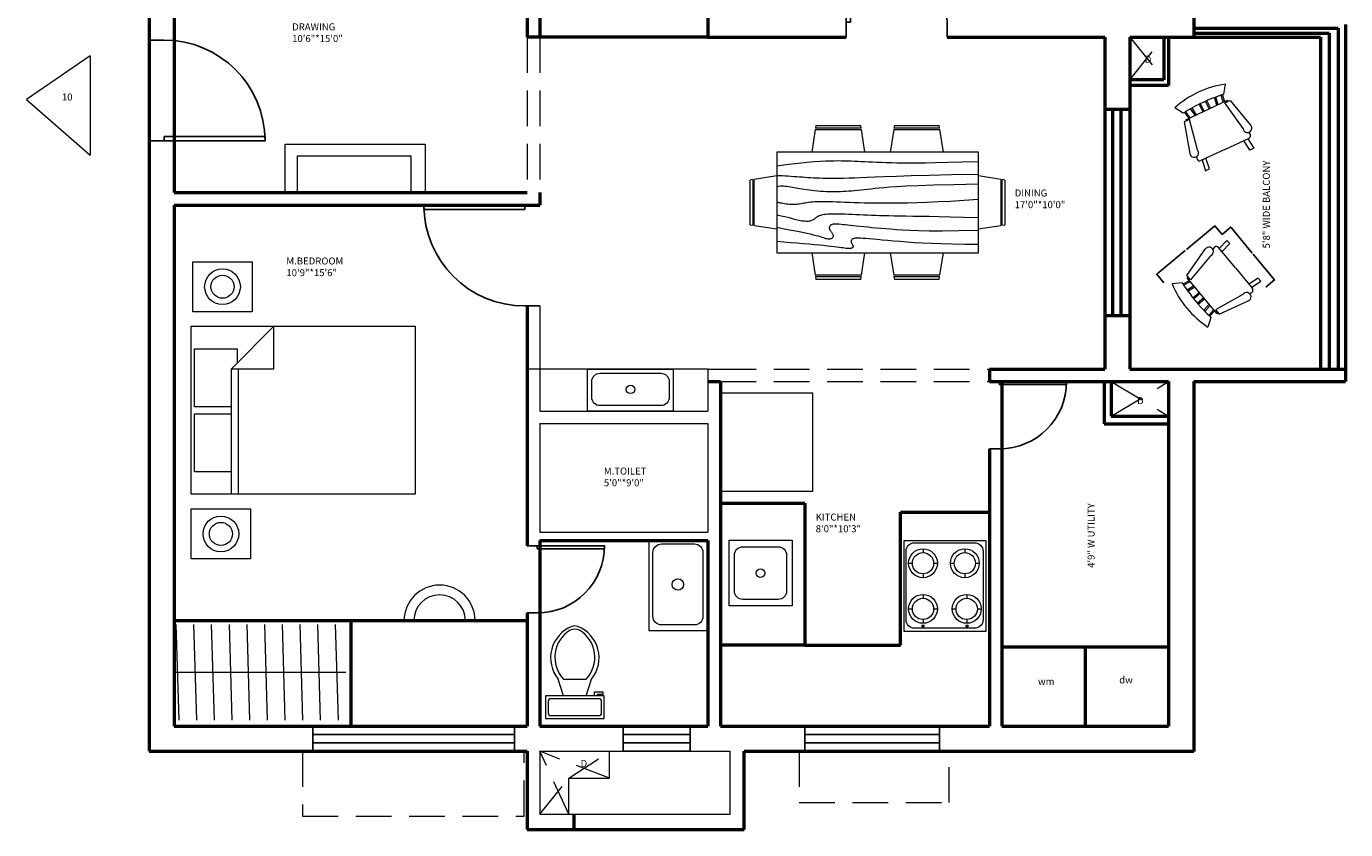
# Model space of a CAD drawing. Units: inches. Extents: x 4795 to 6024, y 2716 to 5025.
# Tile 7 of 19: x 5484 to 5955, y 3324 to 3611. Entities that reach past the tile are written whole.
import ezdxf

# ---------------------------------------------------------------- set-up
doc = ezdxf.new("R2010")
doc.units = ezdxf.units.IN
doc.linetypes.add('DASHED', pattern=[19.05, 12.7, -6.35])
for name, color, linetype, lineweight in [('A-ANNO-DIMS', 2, 'Continuous', 18), ('A-ANNO-TEXT', 7, 'Continuous', 18), ('A-AREA-IDEN', 3, 'Continuous', 18), ('A-DOOR', 4, 'Continuous', 25), ('A-FLOR-FIXT', 9, 'Continuous', 18), ('A-FURN', 8, 'Continuous', 18), ('A-GLAZ', 4, 'Continuous', 25), ('A-WALL', 7, 'Continuous', 50), ('A-WALL-OVHD', 8, 'DASHED', 18)]:
    doc.layers.add(name, color=color, linetype=linetype, lineweight=lineweight)
doc.styles.get("Standard").update_dxf_attribs({"font": 'arial.ttf'})
doc.dimstyles.get("Standard").update_dxf_attribs({"dimtxt": 0.18, "dimasz": 0.18, "dimexe": 0.18, "dimexo": 0.0625, "dimgap": 0.09, "dimtad": 0, "dimtih": 1, "dimtoh": 1, "dimdec": 4, "dimzin": 0, "dimdsep": 46, "dimtxsty": 'Standard', "dimcen": 0.09, "dimadec": 0, "dimazin": 0, "dimtfac": 1, "dimtdec": 4, "dimtofl": 0, "dimtmove": 0, "dimatfit": 3, "dimfxl": 1, "dimtolj": 1, "dimtzin": 0, "dimarcsym": 0})

# ---------------------------------------------------------------- blocks, each defined once
blk = doc.blocks.new('*U2')
for p, q in [((0, 0), (0, -6)), ((40, 0), (40, -6))]:
    blk.add_line(p, q)
blk.add_lwpolyline([(0, 0), (0, 40), (1.75, 40), (1.75, 0)], close=True)
blk.add_arc((0, 0), 40, 0, 90)
blk = doc.blocks.new('Bed - Queen')
for p, q in [((0, -80.00003), (0, 0)), ((0, 0), (59.99999, 0)), ((59.99999, 0), (59.99999, -80.00003)), ((7.99999, -1.2), (28.79998, -1.2)), ((7.99999, -14.4), (7.99999, -1.2)), ((28.79998, -1.2), (28.79998, -14.4)), ((31.19999, -1.2), (51.99999, -1.2)), ((31.19999, -14.4), (31.19999, -1.2)), ((51.99999, -1.2), (51.99999, -16.4)), ((0, -14.4), (44.8, -14.4)), ((44.8, -16.8), (0, -16.8)), ((59.99999, -29.6), (44.8, -14.4)), ((44.8, -14.4), (44.8, -29.6)), ((51.99999, -16.4), (46.79936, -16.4)), ((44.8, -29.6), (59.99999, -29.6)), ((59.99999, -80.00003), (0, -80.00003))]:
    blk.add_line(p, q)
blk = doc.blocks.new('Toilet - top')
for p, q in [((9.5, -6), (9.5, -2)), ((-10, -8.5), (-8, -8.5)), ((-10, -9.5), (-10, -8.5)), ((-8, -8.5), (-8, -8)), ((-7, -8), (-7, -9.5)), ((-4, -8), (-6, -14)), ((4, -8), (6, -14)), ((-7, -9.5), (-10, -9.5)), ((4, -14), (-4, -14))]:
    blk.add_line(p, q)
blk.add_lwpolyline([(10.5, -8), (10.5, 0), (-10.5, 0), (-10.5, -8)], close=True)
for points in [[(-9.5, -2), (-9.5, -6)], [(8.5, -1), (-8.5, -1)], [(-8.5, -7), (8.5, -7)]]:
    blk.add_lwpolyline(points)
for centre, radius, start, end in [((-8.62, -1.88), 0.884, 81.8699, 188.1301), ((8.62, -1.88), 0.884, 351.8699, 98.1301), ((-8.62, -6.12), 0.884, 171.8699, 278.1301), ((8.62, -6.12), 0.884, 261.8699, 8.1301), ((3.52, -21.58), 12.17, 141.4691, 247.9714), ((4.2, -21.82), 11.33, 136.3677, 238.9468), ((-3.52, -21.58), 12.17, 292.0284, 38.5307), ((-4.2, -21.82), 11.33, 301.053, 43.6321), ((0, -27.88), 4, 245.7318, 294.2682), ((0, -29), 4, 254.8605, 285.1395)]:
    blk.add_arc(centre, radius, start, end)
blk = doc.blocks.new('Chair - Rocking')
for p, q in [((-8, -4.5), (-10, -1.5)), ((-7.5, -4.5), (-7, -7)), ((-6.5, -7), (-7.02225, -4.43)), ((-4.5, -7), (-4.96674, -4.19951)), ((-4, -7), (-4.40532, -4.16272)), ((-1.5, -4.05012), (-1.5, -7)), ((-1, -7), (-1, -4.05012)), ((1, -7), (1, -4.04655)), ((1.5, -4.05012), (1.5, -7)), ((4, -7), (4.40187, -4.18694)), ((4.5, -7), (4.96761, -4.19437)), ((6.5, -7), (7, -4.4057)), ((7.5, -4.5), (7, -7)), ((8, -4.5), (10, -1.5)), ((-9, -7.5), (-12, -18.49999)), ((-7, -7.5), (-9, -7.5)), ((-9, -18.49999), (-7, -7.5)), ((-8.23428, -6.99939), (-8.3093, -7.47958)), ((-8.23041, -7), (8.23915, -7)), ((7, -7.5), (9, -7.5)), ((9, -18.49999), (7, -7.5)), ((8.31071, -7.48854), (8.23449, -7.00073)), ((9, -7.5), (12, -18.49999)), ((-10.36644, -20.64523), (-10.5, -21.49999)), ((-9, -22.49999), (-9.5, -26.49999)), ((0, -22.49999), (-9.5, -22.49999)), ((-8, -26.49999), (-7.5, -22.49999)), ((0, -22.49999), (9.5, -22.49999)), ((8, -26.49999), (7.5, -22.49999)), ((9, -22.49999), (9.5, -26.49999)), ((10.5, -21.49999), (10.3575, -20.58798)), ((-9.5, -26.49999), (-8, -26.49999)), ((9.5, -26.49999), (8, -26.49999))]:
    blk.add_line(p, q)
for centre, radius, start, end in [((0, -34.08333), 34.08333, 72.93847, 107.0615), ((0, -68.25004), 64.25, 93.92211, 97.15267), ((0, -68.25004), 64.25, 82.84733, 93.92211), ((-10.5, -18.99999), 1.58114, 161.5651, 18.43495), ((10.5, -18.99999), 1.58114, 161.5651, 18.43495), ((-9.5, -21.49999), 1, 180, 270), ((9.5, -21.49999), 1, 270, 0)]:
    blk.add_arc(centre, radius, start, end)
blk = doc.blocks.new('WIN-48')
for p, q in [((0, 0), (0, 48)), ((0, 48), (9, 48)), ((3, 0), (3, 48)), ((6, 48), (6, 0)), ((9, 48), (9, 0)), ((9, 0), (0, 0))]:
    blk.add_line(p, q)
blk = doc.blocks.new('WIN-72')
for p, q in [((0, 0), (0, 9)), ((0, 9), (72, 9)), ((0, 6), (72, 6)), ((72, 9), (72, 0)), ((72, 3), (0, 3)), ((72, 0), (0, 0))]:
    blk.add_line(p, q)
blk = doc.blocks.new('WIN-24')
for p, q in [((0, 0), (0, 9)), ((0, 9), (24, 9)), ((0, 6), (24, 6)), ((24, 9), (24, 0)), ((24, 3), (0, 3)), ((24, 0), (0, 0))]:
    blk.add_line(p, q)
blk = doc.blocks.new('CHAIR-DINING')
for p, q in [((8, 17.72), (0, 18.97)), ((8, 17.71), (8, 1.25)), ((9.5, 17.48), (8.5, 17.64)), ((8.5, 1.33), (8.5, 17.64)), ((9.5, 17.48), (9.5, 1.48)), ((0, 0), (8, 1.25)), ((8.5, 1.33), (9.5, 1.48))]:
    blk.add_line(p, q)
blk = doc.blocks.new('COOKTOP-4B')
for p, q in [((6.77, 29.57), (6.77, 28.22)), ((21.7, 29.57), (21.7, 28.22)), ((1.61, 24.41), (2.97, 24.41)), ((10.57, 24.41), (11.93, 24.41)), ((16.54, 24.41), (17.9, 24.41)), ((25.51, 24.41), (26.87, 24.41)), ((6.77, 20.61), (6.77, 19.25)), ((21.7, 20.61), (21.7, 19.25)), ((6.77, 13.27), (6.77, 11.91)), ((22.37, 13.27), (22.37, 11.91)), ((1.61, 8.11), (2.97, 8.11)), ((10.57, 8.11), (11.93, 8.11)), ((17.2, 8.11), (18.56, 8.11)), ((26.17, 8.11), (27.53, 8.11)), ((6.77, 4.3), (6.77, 2.94)), ((22.37, 4.3), (22.37, 2.94))]:
    blk.add_line(p, q)
blk.add_lwpolyline([(0, 32.52), (29.24, 32.52), (29.24, 0), (0, 0)], close=True)
blk.add_lwpolyline([(3.72, 31.71), (25.19, 31.71, -0.414214), (28.19, 28.71), (28.19, 4.17, -0.414214), (25.19, 1.17), (3.72, 1.17, -0.414214), (0.72, 4.17), (0.72, 28.71, -0.414214)], format="xyb", close=True)
for centre, radius in [((6.77, 24.41), 5.16), ((21.7, 24.41), 5.16), ((6.77, 24.41), 3.8), ((21.7, 24.41), 3.8), ((6.77, 8.11), 5.16), ((6.77, 8.11), 3.8), ((22.37, 8.11), 5.16), ((22.37, 8.11), 3.8), ((6.77, 2), 0.353), ((22.47, 2), 0.353)]:
    blk.add_circle(centre, radius)
blk = doc.blocks.new('*D39')
at = {"layer": 'A-ANNO-DIMS', "color": 0, "lineweight": -2, "transparency": 16777216}
for p, q in [((5908.61, 3539.46), (5898.58, 3531.14)), ((5911.3, 3536.51), (5908.63, 3539.72)), ((5888.11, 3522.45), (5898.14, 3530.77)), ((5890.52, 3519.26), (5887.86, 3522.47))]:
    blk.add_line(p, q, dxfattribs=at)
at = {"layer": 'A-ANNO-DIMS', "color": 0, "lineweight": 100, "transparency": 16777216}
for points in [[(5908.59, 3539.49), (5908.63, 3539.44), (5908.75, 3539.58)], [(5888.09, 3522.47), (5888.13, 3522.43), (5887.97, 3522.33)]]:
    blk.add_solid(points, dxfattribs=at)
at = {"layer": 'DEFPOINTS', "color": 0, "lineweight": 100, "transparency": 16777216}
for p in [(5911.33, 3536.46), (5887.97, 3522.33), (5890.56, 3519.22)]:
    blk.add_point(p, dxfattribs=at)
at = {"layer": 'A-ANNO-DIMS', "color": 0, "transparency": 16777216, "insert": (5898.36, 3530.96), "char_height": 0.18, "attachment_point": 5}
blk.add_mtext('\\A1;ROCKING CHAIR 27 TYP.', dxfattribs=at)
blk = doc.blocks.new('*D40')
at = {"layer": 'A-ANNO-DIMS', "color": 0, "lineweight": -2, "transparency": 16777216}
for p, q in [((5911.38, 3536.5), (5914.59, 3539.16)), ((5914.57, 3538.91), (5922.1, 3529.83)), ((5929.94, 3520.39), (5922.4, 3529.47)), ((5926.99, 3517.7), (5930.2, 3520.36))]:
    blk.add_line(p, q, dxfattribs=at)
at = {"layer": 'A-ANNO-DIMS', "color": 0, "lineweight": 100, "transparency": 16777216}
for points in [[(5914.59, 3538.93), (5914.54, 3538.89), (5914.45, 3539.05)], [(5929.97, 3520.41), (5929.92, 3520.37), (5930.06, 3520.25)]]:
    blk.add_solid(points, dxfattribs=at)
at = {"layer": 'DEFPOINTS', "color": 0, "lineweight": 100, "transparency": 16777216}
for p in [(5914.45, 3539.05), (5911.33, 3536.46), (5926.94, 3517.66)]:
    blk.add_point(p, dxfattribs=at)
at = {"layer": 'A-ANNO-DIMS', "color": 0, "transparency": 16777216, "insert": (5922.25, 3529.65), "char_height": 0.18, "attachment_point": 5}
blk.add_mtext('\\A1;24 TYP.', dxfattribs=at)

msp = doc.modelspace()

# ---------------------------------------------------------------- linework, layer by layer
at = {"layer": 'A-FLOR-FIXT'}
for points in [[(5684.77, 3488.43), (5715.33, 3488.43), (5715.33, 3473.43), (5684.77, 3473.43)], [(5735.36, 3427.32), (5757.88, 3427.32), (5757.88, 3403.85), (5735.36, 3403.85)]]:
    msp.add_lwpolyline(points, close=True, dxfattribs=at)
for points in [[(5689.26, 3486.93), (5710.91, 3486.93, -0.414214), (5713.91, 3483.93), (5713.91, 3478.34, -0.414214), (5710.91, 3475.34), (5689.26, 3475.34, -0.414214), (5686.26, 3478.34), (5686.26, 3483.93, -0.414214)], [(5740.23, 3424.98), (5752.81, 3424.98, -0.414214), (5755.81, 3421.98), (5755.81, 3409.15, -0.414214), (5752.81, 3406.15), (5740.23, 3406.15, -0.414214), (5737.23, 3409.15), (5737.23, 3421.98, -0.414214)]]:
    msp.add_lwpolyline(points, format="xyb", close=True, dxfattribs=at)
for centre, radius in [((5700.08, 3481.14), 1.51), ((5746.52, 3415.57), 1.54)]:
    msp.add_circle(centre, radius, dxfattribs=at)
at = {"layer": 'A-FURN'}
for p, q in [((5507.23, 3600.24), (5484.41, 3584.7)), ((5507.23, 3600.24), (5507.23, 3564.8)), ((5484.41, 3584.7), (5507.23, 3564.8)), ((5576.76, 3551.43), (5576.76, 3568.73)), ((5576.76, 3568.73), (5626.76, 3568.73)), ((5626.76, 3568.73), (5626.76, 3551.43)), ((5824.31, 3565.91), (5752.31, 3565.91)), ((5752.31, 3565.91), (5752.31, 3529.91)), ((5824.31, 3529.91), (5824.31, 3565.91)), ((5581.26, 3551.43), (5581.26, 3564.5)), ((5581.26, 3564.5), (5621.64, 3564.5)), ((5621.64, 3564.5), (5621.64, 3551.43)), ((5752.31, 3557.4), (5744.31, 3556.14)), ((5743.81, 3556.07), (5742.81, 3555.91)), ((5742.81, 3539.91), (5742.81, 3555.91)), ((5743.81, 3556.07), (5743.81, 3539.76)), ((5744.31, 3539.68), (5744.31, 3556.15)), ((5742.81, 3539.91), (5743.81, 3539.75)), ((5744.31, 3539.68), (5752.31, 3538.43)), ((5752.31, 3529.91), (5824.31, 3529.91)), ((5667.72, 3510.93), (5667.72, 3473.43)), ((5727.72, 3488.43), (5663.22, 3488.43)), ((5727.72, 3488.43), (5727.72, 3473.43)), ((5727.72, 3488.43), (5732.22, 3488.43)), ((5667.72, 3473.43), (5727.72, 3473.43)), ((5667.72, 3468.93), (5727.72, 3468.93)), ((5667.72, 3468.93), (5667.72, 3430.16)), ((5727.72, 3468.93), (5727.72, 3430.16)), ((5667.72, 3430.16), (5727.72, 3430.16)), ((5538.93, 3363.05), (5537.92, 3397.25)), ((5545.25, 3363.05), (5544.24, 3397.25)), ((5551.56, 3363.05), (5550.55, 3397.25)), ((5557.88, 3363.05), (5556.87, 3397.25)), ((5564.2, 3363.05), (5563.19, 3397.25)), ((5570.52, 3363.05), (5569.51, 3397.25)), ((5576.84, 3363.05), (5575.83, 3397.25)), ((5583.16, 3363.05), (5582.15, 3397.25)), ((5589.47, 3363.05), (5588.47, 3397.25)), ((5595.79, 3363.05), (5594.78, 3397.25)), ((5537.74, 3380.15), (5598.49, 3380.15)), ((5667.72, 3351.93), (5667.72, 3329.49)), ((5667.72, 3351.93), (5735.65, 3351.93)), ((5692.65, 3342.28), (5692.65, 3351.93)), ((5735.65, 3329.49), (5735.65, 3351.93)), ((5678.06, 3329.49), (5678.06, 3342.28)), ((5678.06, 3342.28), (5692.65, 3342.28)), ((5667.72, 3329.49), (5735.65, 3329.49))]:
    msp.add_line(p, q, dxfattribs=at)
for points in [[(5824.31, 3562.41), (5818.4, 3562.25), (5813.35, 3562.12), (5809.04, 3562.04), (5805.39, 3561.98), (5802.28, 3561.96), (5799.61, 3561.95), (5797.28, 3561.97), (5795.19, 3561.99), (5793.23, 3562.03), (5791.4, 3562.07), (5789.68, 3562.12), (5788.07, 3562.17), (5786.55, 3562.23), (5785.11, 3562.29), (5783.76, 3562.35), (5782.48, 3562.41), (5781.26, 3562.47), (5780.08, 3562.53), (5778.92, 3562.59), (5777.77, 3562.63), (5776.59, 3562.67), (5775.38, 3562.7), (5774.12, 3562.71), (5772.77, 3562.7), (5771.32, 3562.67), (5769.7, 3562.62), (5767.83, 3562.51), (5765.65, 3562.35), (5763.08, 3562.13), (5760.05, 3561.82), (5756.48, 3561.42), (5752.31, 3560.91)], [(5824.31, 3557.91), (5814.71, 3557.72), (5806.78, 3557.54), (5800.3, 3557.36), (5795.05, 3557.19), (5790.83, 3557.03), (5787.43, 3556.89), (5784.64, 3556.77), (5782.23, 3556.66), (5780.04, 3556.58), (5778.01, 3556.52), (5776.14, 3556.48), (5774.42, 3556.45), (5772.82, 3556.44), (5771.35, 3556.45), (5769.99, 3556.47), (5768.73, 3556.49), (5767.55, 3556.53), (5766.44, 3556.57), (5765.39, 3556.62), (5764.38, 3556.68), (5763.4, 3556.74), (5762.44, 3556.8), (5761.47, 3556.88), (5760.48, 3556.95), (5759.46, 3557.03), (5758.43, 3557.11), (5757.38, 3557.19), (5756.33, 3557.26), (5755.29, 3557.32), (5754.27, 3557.37), (5753.27, 3557.4), (5752.31, 3557.41)], [(5824.31, 3554.41), (5815.5, 3554.22), (5808.4, 3554.04), (5802.78, 3553.85), (5798.42, 3553.67), (5795.09, 3553.49), (5792.55, 3553.32), (5790.57, 3553.15), (5788.94, 3552.99), (5787.44, 3552.84), (5786.04, 3552.7), (5784.72, 3552.56), (5783.48, 3552.43), (5782.31, 3552.31), (5781.18, 3552.2), (5780.11, 3552.09), (5779.06, 3551.99), (5778.04, 3551.9), (5777.04, 3551.82), (5776.05, 3551.76), (5775.06, 3551.7), (5774.08, 3551.66), (5773.09, 3551.64), (5772.08, 3551.64), (5771.06, 3551.66), (5770.02, 3551.7), (5768.97, 3551.77), (5767.91, 3551.85), (5766.86, 3551.94), (5765.84, 3552.05), (5764.84, 3552.16), (5763.88, 3552.29), (5762.98, 3552.41), (5762.13, 3552.54), (5761.34, 3552.66), (5760.6, 3552.78), (5759.89, 3552.91), (5759.21, 3553.03), (5758.55, 3553.14), (5757.91, 3553.26), (5757.27, 3553.37), (5756.63, 3553.47), (5755.99, 3553.57), (5755.35, 3553.64), (5754.71, 3553.69), (5754.09, 3553.69), (5753.48, 3553.66), (5752.89, 3553.56), (5752.31, 3553.41)], [(5824.31, 3548.91), (5819.1, 3548.57), (5814.33, 3548.29), (5809.96, 3548.07), (5805.97, 3547.91), (5802.31, 3547.78), (5798.96, 3547.7), (5795.89, 3547.65), (5793.06, 3547.62), (5790.45, 3547.61), (5788.02, 3547.62), (5785.78, 3547.65), (5783.7, 3547.69), (5781.76, 3547.73), (5779.95, 3547.79), (5778.25, 3547.85), (5776.65, 3547.91), (5775.12, 3547.97), (5773.68, 3548.03), (5772.31, 3548.08), (5771.03, 3548.13), (5769.83, 3548.16), (5768.71, 3548.18), (5767.68, 3548.18), (5766.73, 3548.16), (5765.86, 3548.12), (5765.08, 3548.06), (5764.36, 3547.98), (5763.7, 3547.89), (5763.09, 3547.79), (5762.52, 3547.69), (5761.99, 3547.59), (5761.48, 3547.49), (5760.99, 3547.4), (5760.5, 3547.32), (5760.02, 3547.26), (5759.54, 3547.2), (5759.05, 3547.16), (5758.55, 3547.14), (5758.03, 3547.14), (5757.48, 3547.16), (5756.9, 3547.2), (5756.31, 3547.26), (5755.72, 3547.34), (5755.15, 3547.42), (5754.61, 3547.51), (5754.12, 3547.59), (5753.7, 3547.67), (5753.35, 3547.74), (5753.1, 3547.8), (5752.93, 3547.84), (5752.81, 3547.87), (5752.72, 3547.89), (5752.65, 3547.9), (5752.57, 3547.91), (5752.47, 3547.91), (5752.31, 3547.91)], [(5824.31, 3542.41), (5819.03, 3542.58), (5814.38, 3542.7), (5810.31, 3542.79), (5806.74, 3542.86), (5803.61, 3542.9), (5800.86, 3542.94), (5798.42, 3542.97), (5796.23, 3542.99), (5794.22, 3543.03), (5792.37, 3543.07), (5790.65, 3543.12), (5789.05, 3543.17), (5787.54, 3543.23), (5786.09, 3543.29), (5784.69, 3543.35), (5783.31, 3543.41), (5781.94, 3543.47), (5780.58, 3543.53), (5779.24, 3543.59), (5777.94, 3543.64), (5776.68, 3543.68), (5775.48, 3543.71), (5774.36, 3543.74), (5773.31, 3543.74), (5772.36, 3543.74), (5771.49, 3543.71), (5770.71, 3543.67), (5770.01, 3543.62), (5769.38, 3543.55), (5768.82, 3543.46), (5768.33, 3543.36), (5767.9, 3543.24), (5767.52, 3543.11), (5767.18, 3542.97), (5766.89, 3542.81), (5766.62, 3542.65), (5766.38, 3542.48), (5766.16, 3542.32), (5765.94, 3542.15), (5765.73, 3541.99), (5765.51, 3541.84), (5765.27, 3541.7), (5765.02, 3541.57), (5764.76, 3541.45), (5764.48, 3541.35), (5764.17, 3541.27), (5763.84, 3541.2), (5763.48, 3541.16), (5763.09, 3541.14), (5762.67, 3541.14), (5762.23, 3541.17), (5761.76, 3541.21), (5761.27, 3541.28), (5760.77, 3541.36), (5760.26, 3541.46), (5759.73, 3541.58), (5759.19, 3541.71), (5758.6, 3541.86), (5757.95, 3542.04), (5757.18, 3542.24), (5756.26, 3542.48), (5755.17, 3542.75), (5753.86, 3543.06), (5752.31, 3543.41)], [(5824.31, 3537.91), (5817.29, 3537.77), (5811.48, 3537.71), (5806.74, 3537.71), (5802.88, 3537.77), (5799.75, 3537.88), (5797.19, 3538.02), (5795.03, 3538.17), (5793.1, 3538.33), (5791.28, 3538.48), (5789.54, 3538.63), (5787.87, 3538.76), (5786.29, 3538.9), (5784.79, 3539.03), (5783.37, 3539.16), (5782.05, 3539.29), (5780.81, 3539.41), (5779.67, 3539.53), (5778.62, 3539.66), (5777.66, 3539.77), (5776.78, 3539.88), (5775.99, 3539.97), (5775.27, 3540.05), (5774.63, 3540.12), (5774.06, 3540.16), (5773.56, 3540.18), (5773.13, 3540.18), (5772.76, 3540.15), (5772.44, 3540.11), (5772.16, 3540.04), (5771.93, 3539.96), (5771.73, 3539.86), (5771.56, 3539.74), (5771.42, 3539.61), (5771.3, 3539.46), (5771.2, 3539.31), (5771.13, 3539.14), (5771.09, 3538.96), (5771.08, 3538.78), (5771.1, 3538.6), (5771.15, 3538.41), (5771.22, 3538.22), (5771.32, 3538.04), (5771.45, 3537.85), (5771.58, 3537.66), (5771.73, 3537.47), (5771.87, 3537.29), (5772.01, 3537.1), (5772.15, 3536.91), (5772.26, 3536.72), (5772.36, 3536.54), (5772.44, 3536.35), (5772.49, 3536.17), (5772.51, 3535.99), (5772.51, 3535.82), (5772.47, 3535.65), (5772.4, 3535.49), (5772.28, 3535.34), (5772.13, 3535.2), (5771.95, 3535.08), (5771.74, 3534.97), (5771.5, 3534.89), (5771.24, 3534.84), (5770.95, 3534.81), (5770.65, 3534.83), (5770.32, 3534.88), (5769.97, 3534.96), (5769.57, 3535.08), (5769.12, 3535.23), (5768.59, 3535.4), (5767.98, 3535.59), (5767.27, 3535.81), (5766.44, 3536.04), (5765.48, 3536.28), (5764.35, 3536.54), (5763.03, 3536.82), (5761.48, 3537.14), (5759.67, 3537.51), (5757.56, 3537.92), (5755.12, 3538.38), (5752.31, 3538.91)], [(5824.31, 3532.91), (5819.49, 3532.93), (5815.12, 3533), (5811.17, 3533.09), (5807.59, 3533.22), (5804.35, 3533.37), (5801.41, 3533.54), (5798.73, 3533.72), (5796.27, 3533.91), (5794, 3534.1), (5791.92, 3534.28), (5790.01, 3534.46), (5788.28, 3534.62), (5786.72, 3534.77), (5785.33, 3534.89), (5784.11, 3535), (5783.06, 3535.08), (5782.17, 3535.12), (5781.43, 3535.14), (5780.82, 3535.13), (5780.33, 3535.1), (5779.94, 3535.04), (5779.64, 3534.96), (5779.41, 3534.86), (5779.23, 3534.74), (5779.09, 3534.61), (5778.99, 3534.47), (5778.92, 3534.31), (5778.88, 3534.15), (5778.87, 3533.98), (5778.89, 3533.82), (5778.92, 3533.65), (5778.98, 3533.49), (5779.05, 3533.34), (5779.13, 3533.2), (5779.21, 3533.06), (5779.3, 3532.92), (5779.38, 3532.79), (5779.46, 3532.66), (5779.52, 3532.54), (5779.56, 3532.41), (5779.58, 3532.29), (5779.58, 3532.16), (5779.55, 3532.04), (5779.5, 3531.93), (5779.43, 3531.83), (5779.33, 3531.73), (5779.21, 3531.65), (5779.06, 3531.58), (5778.89, 3531.52), (5778.69, 3531.48), (5778.46, 3531.46), (5778.19, 3531.45), (5777.87, 3531.46), (5777.49, 3531.48), (5777.06, 3531.52), (5776.56, 3531.58), (5775.99, 3531.65), (5775.34, 3531.73), (5774.6, 3531.83), (5773.74, 3531.94), (5772.77, 3532.06), (5771.67, 3532.2), (5770.42, 3532.34), (5769.02, 3532.49), (5767.45, 3532.65), (5765.72, 3532.82), (5763.84, 3532.99), (5761.81, 3533.17), (5759.63, 3533.35), (5757.32, 3533.54), (5754.88, 3533.72), (5752.31, 3533.91)]]:
    msp.add_lwpolyline(points, dxfattribs=at)
for points in [[(5543.79, 3526.72), (5565.06, 3526.72), (5565.06, 3508.89), (5543.79, 3508.89)], [(5732.22, 3444.76), (5765.22, 3444.76), (5765.22, 3479.81), (5732.22, 3479.81)], [(5543.21, 3438.47), (5564.48, 3438.47), (5564.48, 3420.63), (5543.21, 3420.63)], [(5727.72, 3427.25), (5706.66, 3427.25), (5706.66, 3395.02), (5727.72, 3395.02)]]:
    msp.add_lwpolyline(points, close=True, dxfattribs=at)
msp.add_lwpolyline([(5711.13, 3425.96), (5722.94, 3425.96, -0.414214), (5725.94, 3422.96), (5725.94, 3400.05, -0.414214), (5722.94, 3397.05), (5711.13, 3397.05, -0.414214), (5708.13, 3400.05), (5708.13, 3422.96, -0.414214)], format="xyb", close=True, dxfattribs=at)
for centre, radius in [((5554.43, 3517.81), 6.37), ((5554.43, 3517.81), 4.11), ((5553.85, 3429.55), 6.37), ((5553.85, 3429.55), 4.11), ((5717.03, 3411.5), 2.04)]:
    msp.add_circle(centre, radius, dxfattribs=at)
for radius in [12.67, 9.2]:
    msp.add_arc((5631.95, 3398.59), radius, 360, 180, dxfattribs=at)
at = {"layer": 'A-WALL'}
for p, q in [((5528.22, 3920.81), (5528.22, 3351.93)), ((5901.22, 3740.43), (5901.22, 3606.93)), ((5537.22, 3731.43), (5537.22, 3551.43)), ((5663.22, 3731.43), (5663.22, 3606.93)), ((5667.72, 3624.93), (5667.72, 3606.93)), ((5727.72, 3624.93), (5727.72, 3606.93)), ((5901.22, 3610.12), (5952.78, 3610.12)), ((5901.22, 3608.31), (5949.55, 3608.31)), ((5949.55, 3608.31), (5949.55, 3488.43)), ((5952.78, 3610.12), (5952.78, 3488.43)), ((5955.43, 3611.43), (5955.43, 3483.93)), ((5727.72, 3606.93), (5663.22, 3606.93)), ((5727.72, 3606.93), (5777.13, 3606.93)), ((5813.13, 3606.93), (5869.43, 3606.93)), ((5869.43, 3606.93), (5869.43, 3488.43)), ((5878.43, 3606.93), (5878.43, 3488.43)), ((5878.43, 3606.93), (5901.22, 3606.93)), ((5890.54, 3606.93), (5890.54, 3591.73)), ((5892.22, 3606.93), (5892.22, 3589.64)), ((5901.22, 3606.93), (5946.43, 3606.93)), ((5946.43, 3606.93), (5946.43, 3488.43)), ((5890.54, 3591.73), (5878.43, 3591.73)), ((5892.22, 3589.64), (5878.43, 3589.64)), ((5869.43, 3581.18), (5878.43, 3581.18)), ((5872.23, 3581.18), (5872.23, 3507.48)), ((5875.16, 3581.18), (5875.16, 3507.48)), ((5537.22, 3551.43), (5663.22, 3551.43)), ((5537.22, 3546.93), (5667.72, 3546.93)), ((5537.22, 3546.93), (5537.22, 3360.93)), ((5667.72, 3551.43), (5667.72, 3546.93)), ((5663.22, 3510.93), (5663.22, 3425.32)), ((5869.43, 3507.48), (5878.43, 3507.48)), ((5828.22, 3488.43), (5828.22, 3483.93)), ((5828.22, 3488.43), (5869.43, 3488.43)), ((5878.43, 3488.43), (5901.22, 3488.43)), ((5901.22, 3488.43), (5955.43, 3488.43)), ((5727.72, 3483.93), (5732.22, 3483.93)), ((5732.22, 3483.93), (5732.22, 3360.93)), ((5828.22, 3483.93), (5892.22, 3483.93)), ((5832.72, 3483.93), (5832.72, 3360.93)), ((5869.22, 3483.93), (5869.22, 3468.81)), ((5871.76, 3483.93), (5871.76, 3471.62)), ((5892.22, 3483.93), (5892.22, 3360.93)), ((5901.22, 3483.93), (5901.22, 3351.9)), ((5901.22, 3483.93), (5955.43, 3483.93)), ((5871.76, 3471.62), (5892.22, 3471.62)), ((5869.22, 3468.81), (5892.22, 3468.81)), ((5828.22, 3459.93), (5828.22, 3360.93)), ((5732.22, 3440.48), (5762.33, 3440.48)), ((5762.33, 3440.48), (5762.33, 3389.86)), ((5796.52, 3389.86), (5796.52, 3437.35)), ((5796.52, 3437.35), (5828.22, 3437.35)), ((5667.72, 3427.25), (5667.72, 3360.93)), ((5667.72, 3427.25), (5706.66, 3427.25)), ((5706.66, 3427.25), (5727.72, 3427.25)), ((5727.72, 3427.25), (5727.72, 3360.93)), ((5663.22, 3401.32), (5663.22, 3360.93)), ((5537.22, 3398.59), (5663.22, 3398.59)), ((5600.22, 3398.59), (5600.22, 3360.93)), ((5762.33, 3389.86), (5732.22, 3389.86)), ((5762.33, 3389.86), (5796.52, 3389.86)), ((5832.72, 3389.21), (5892.22, 3389.21)), ((5862.47, 3389.21), (5862.47, 3360.93)), ((5537.22, 3360.93), (5663.22, 3360.93)), ((5667.72, 3360.93), (5727.72, 3360.93)), ((5732.22, 3360.93), (5828.22, 3360.93)), ((5832.72, 3360.93), (5892.22, 3360.93)), ((5528.22, 3351.93), (5663.22, 3351.93)), ((5537.22, 3351.93), (5537.22, 3351.9)), ((5663.22, 3351.93), (5663.22, 3323.95)), ((5740.64, 3323.95), (5740.64, 3351.93)), ((5740.64, 3351.93), (5901.22, 3351.93)), ((5892.22, 3351.93), (5892.22, 3351.9)), ((5679.92, 3329.49), (5679.92, 3323.95)), ((5663.22, 3323.95), (5740.64, 3323.95))]:
    msp.add_line(p, q, dxfattribs=at)
at = {"layer": 'A-WALL-OVHD'}
for p, q in [((5663.22, 3606.93), (5663.22, 3551.43)), ((5667.72, 3606.93), (5667.72, 3551.43)), ((5878.43, 3606.93), (5890.54, 3591.73)), ((5878.43, 3591.73), (5890.54, 3606.93)), ((5732.22, 3488.43), (5828.22, 3488.43)), ((5732.22, 3483.93), (5828.22, 3483.93)), ((5871.76, 3483.93), (5892.22, 3471.62)), ((5871.76, 3471.62), (5892.22, 3483.93)), ((5582.99, 3351.93), (5582.99, 3328.81)), ((5662.13, 3328.81), (5662.13, 3351.93)), ((5678.06, 3329.49), (5667.72, 3351.93)), ((5692.65, 3342.28), (5667.72, 3351.93)), ((5678.06, 3342.28), (5692.65, 3351.93)), ((5760.3, 3351.93), (5760.3, 3333.59)), ((5813.89, 3333.59), (5813.89, 3351.93)), ((5667.72, 3329.49), (5678.06, 3342.28)), ((5760.3, 3333.59), (5813.89, 3333.59)), ((5582.99, 3328.81), (5662.13, 3328.81))]:
    msp.add_line(p, q, dxfattribs=at)

# ---------------------------------------------------------------- block references
at = {"layer": 'A-DOOR', "xscale": 0.9, "yscale": 0.9, "zscale": 0.9}
msp.add_blockref('*U2', (5777.13, 3612.33), dxfattribs=at)
at = {"layer": 'A-DOOR'}
for p, xscale, yscale, zscale, rotation in [((5533.62, 3569.87), -0.9, 0.9, 0.9, 270), ((5662.32, 3546.93), -0.9, 0.9, 0.9, 90), ((5831.82, 3483.93), 0.6, 0.6, 0.6, 270), ((5666.82, 3425.32), 0.6, 0.6, 0.6, 270)]:
    msp.add_blockref('*U2', p, dxfattribs=dict(at, xscale=xscale, yscale=yscale, zscale=zscale, rotation=rotation))
at = {"layer": 'A-FLOR-FIXT'}
msp.add_blockref('COOKTOP-4B', (5797.77, 3394.67), dxfattribs=at)
at = {"layer": 'A-FLOR-FIXT', "rotation": 180}
msp.add_blockref('Toilet - top', (5680.23, 3363.67), dxfattribs=at)
at = {"layer": 'A-FURN'}
for name, p, rotation in [('Chair - Rocking', (5902.83, 3587.26), 24.98478846597024), ('CHAIR-DINING', (5783.8, 3565.91), 90.0056718244202), ('CHAIR-DINING', (5811.8, 3565.91), 90.0056718244202), ('CHAIR-DINING', (5824.31, 3538.43), 0.0068516407015718), ('Chair - Rocking', (5898.75, 3510.14), 129.6958839725731), ('CHAIR-DINING', (5764.83, 3529.91), 270.0000000000017), ('CHAIR-DINING', (5792.83, 3529.91), 270.0000000000017), ('Bed - Queen', (5543.21, 3443.68), 90)]:
    msp.add_blockref(name, p, dxfattribs=dict(at, rotation=rotation))
at = {"layer": 'A-GLAZ'}
for name, p, rotation in [('WIN-72', (5658.72, 3360.93), 180), ('WIN-24', (5721.45, 3360.93), 180), ('WIN-48', (5810.37, 3351.93), 90.00000000000183)]:
    msp.add_blockref(name, p, dxfattribs=dict(at, rotation=rotation))

# ---------------------------------------------------------------- texts
at = {"layer": 'A-ANNO-TEXT', "char_height": 2.5, "attachment_point": 1}
for s, width, insert in [('D', 1.7542, (5883.73, 3600.28)), ('10', 9.3642, (5497.09, 3586.81)), ('D', 2.1417, (5880.99, 3478.38)), ('wm', 19.6889, (5845.59, 3378.11)), ('dw', 16.3455, (5874.6, 3378.67)), ('D', 2.5724, (5682.29, 3348.82))]:
    msp.add_mtext_dynamic_manual_height_columns(s, width=width, gutter_width=12.5, heights=[0], dxfattribs=dict(at, insert=insert))
at = {"layer": 'A-AREA-IDEN', "char_height": 2.5, "attachment_point": 1}
for s, width, insert in [('DRAWING\\P10\'6"*15\'0"', 61.2488, (5579.3, 3611.86)), ('DINING\\P17\'0"*10\'0"', 27.2168, (5837.27, 3552.53)), ('M.BEDROOM\\P10\'9"*15\'6"', 47.3467, (5577.24, 3528.25)), ('M.TOILET\\P5\'0"*9\'0"', 46.3197, (5690.6, 3453.23)), ('KITCHEN\\P8\'0"*10\'3"', 26.7293, (5766.22, 3436.81))]:
    msp.add_mtext_dynamic_manual_height_columns(s, width=width, gutter_width=12.5, heights=[0], dxfattribs=dict(at, insert=insert))
at = {"layer": 'A-AREA-IDEN', "char_height": 2.5, "attachment_point": 1, "rotation": 90}
for s, width, insert in [('5\'8" WIDE BALCONY', 44.4289, (5925.87, 3531.48)), ('4\'9" W UTILITY', 47.405, (5863.29, 3417.42))]:
    msp.add_mtext_dynamic_manual_height_columns(s, width=width, gutter_width=12.5, heights=[0], dxfattribs=dict(at, insert=insert))

# ---------------------------------------------------------------- dimensions: what is measured, and where the dimension line sits
at = {"layer": 'A-ANNO-DIMS'}
for base, p1, p2, angle, text, picture, middle in [((5887.97, 3522.33), (5911.33, 3536.46), (5890.56, 3519.22), 219.6959, 'ROCKING CHAIR <> TYP.', '*D39', (5898.36, 3530.96)), ((5914.45, 3539.05), (5926.94, 3517.66), (5911.33, 3536.46), 129.6959, '<> TYP.', '*D40', (5922.25, 3529.65))]:
    dim = msp.add_linear_dim(base=base, p1=p1, p2=p2, angle=angle, text=text, dimstyle='Standard', override={"dimdec": 0, "dimlfac": 1, "dimrnd": 0, "dimzin": 0, "dimdsep": 46, "dimlunit": 2}, dxfattribs=at)
    dim.commit()
    dim.dimension.update_dxf_attribs({"geometry": picture, "text_midpoint": middle})

doc.saveas('drawing.dxf')
